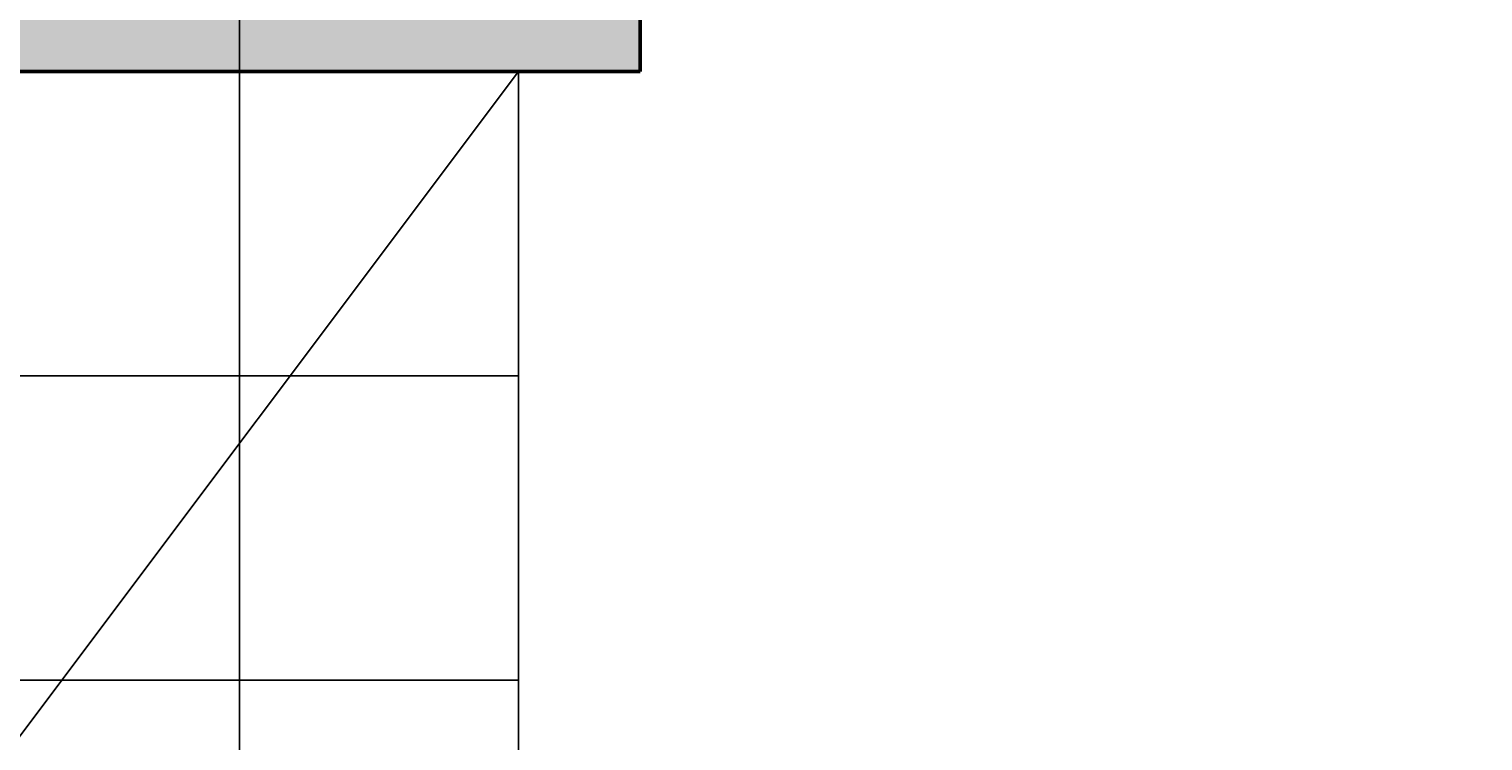
# Model space of a CAD drawing. Units: inches. Extents: x 2231 to 2461, y 2045 to 2455.
# Tile 7 of 95: x 2279 to 2326, y 2099 to 2122. Entities that reach past the tile are written whole.
import ezdxf

# ---------------------------------------------------------------- set-up
doc = ezdxf.new("R2010")
doc.units = ezdxf.units.IN
for name, color, linetype, lineweight in [('A-ANNO-DIMS', 2, 'Continuous', 18), ('A-FLOR-EVTR', 8, 'Continuous', 25), ('A-WALL', 7, 'Continuous', 50)]:
    doc.layers.add(name, color=color, linetype=linetype, lineweight=lineweight)
doc.layers.add('A-WALL-PATT', color=18, linetype='Continuous', lineweight=13, true_color=0x000000)
doc.styles.get("Standard").update_dxf_attribs({"font": 'arial.ttf'})
doc.dimstyles.get("Standard").update_dxf_attribs({"dimtxt": 0.18, "dimasz": 0.18, "dimexe": 0.18, "dimexo": 0.0625, "dimgap": 0.09, "dimtad": 0, "dimtih": 1, "dimtoh": 1, "dimdec": 4, "dimzin": 0, "dimdsep": 46, "dimtxsty": 'Standard', "dimcen": 0.09, "dimadec": 0, "dimazin": 0, "dimtfac": 1, "dimtdec": 4, "dimtofl": 0, "dimtmove": 0, "dimatfit": 3, "dimfxl": 1, "dimtolj": 1, "dimtzin": 0, "dimarcsym": 0})

# ---------------------------------------------------------------- blocks, each defined once
blk = doc.blocks.new('*D51')
at = {"layer": 'A-ANNO-DIMS', "color": 0, "lineweight": -2, "transparency": 16777216}
for p, q in [((2258.794, 2306.77), (2258.794, 2044.803)), ((2330.794, 2306.77), (2330.794, 2044.803)), ((2258.974, 2044.983), (2294.576, 2044.983)), ((2330.614, 2044.983), (2295.011, 2044.983))]:
    blk.add_line(p, q, dxfattribs=at)
at = {"layer": 'A-ANNO-DIMS', "color": 0, "transparency": 16777216}
for points in [[(2258.974, 2045.013), (2258.974, 2044.953), (2258.794, 2044.983)], [(2330.614, 2045.013), (2330.614, 2044.953), (2330.794, 2044.983)]]:
    blk.add_solid(points, dxfattribs=at)
at = {"layer": 'Defpoints', "color": 0, "transparency": 16777216}
for p in [(2258.794, 2306.833), (2330.794, 2306.833), (2330.794, 2044.983)]:
    blk.add_point(p, dxfattribs=at)
at = {"layer": 'A-ANNO-DIMS', "color": 0, "transparency": 16777216, "insert": (2294.794, 2044.983), "char_height": 0.18, "attachment_point": 5}
blk.add_mtext('\\A1;72', dxfattribs=at)
blk = doc.blocks.new('*D65')
at = {"layer": 'A-ANNO-DIMS', "color": 0, "lineweight": -2, "transparency": 16777216}
for p, q in [((2285.635, 2189.285), (2285.635, 2044.803)), ((2340.667, 2189.285), (2340.667, 2044.803)), ((2285.815, 2044.983), (2312.758, 2044.983)), ((2340.487, 2044.983), (2313.545, 2044.983))]:
    blk.add_line(p, q, dxfattribs=at)
at = {"layer": 'A-ANNO-DIMS', "color": 0, "transparency": 16777216}
for points in [[(2285.815, 2045.013), (2285.815, 2044.953), (2285.635, 2044.983)], [(2340.487, 2045.013), (2340.487, 2044.953), (2340.667, 2044.983)]]:
    blk.add_solid(points, dxfattribs=at)
at = {"layer": 'Defpoints', "color": 0, "transparency": 16777216}
for p in [(2285.635, 2189.348), (2340.667, 2189.348), (2340.667, 2044.983)]:
    blk.add_point(p, dxfattribs=at)
at = {"layer": 'A-ANNO-DIMS', "color": 0, "transparency": 16777216, "insert": (2313.151, 2044.983), "char_height": 0.18, "attachment_point": 5}
blk.add_mtext('\\A1;55.03', dxfattribs=at)

msp = doc.modelspace()

# ---------------------------------------------------------------- hatches: boundary and pattern name
at = {"layer": 'A-WALL-PATT'}
h = msp.add_hatch(color=256, dxfattribs=at)
h.dxf.hatch_style = 1
h.paths.add_polyline_path([(2441.7935, 2269.1535), (2432.7935, 2269.1535), (2432.7935, 2186.8328), (2396.7935, 2186.8328), (2396.7935, 2286.8328), (2394.7935, 2286.8328), (2394.7935, 2186.8328), (2334.7935, 2186.8328), (2334.7935, 2182.8328), (2432.7935, 2182.8328), (2432.7935, 2072.8328), (2416.6639, 2072.8328), (2416.6639, 2063.8328), (2441.7935, 2063.8328)])
h.paths.add_polyline_path([(2368.6639, 2072.8328), (2367.04, 2072.8328), (2330.7942, 2072.8328), (2330.7397, 2063.8328), (2368.6639, 2063.8328)])
h.paths.add_polyline_path([(2300.7392, 2068.3328), (2300.7392, 2072.8328), (2298.7935, 2072.8328), (2294.7935, 2072.8328), (2258.7935, 2072.8328), (2258.7935, 2120.8328), (2294.7935, 2120.8328), (2298.7935, 2120.8328), (2298.7935, 2128.8328), (2294.7935, 2128.8328), (2294.7935, 2124.8328), (2258.7935, 2124.8328), (2258.7935, 2182.8328), (2294.7935, 2182.8328), (2294.7935, 2174.8328), (2298.7935, 2174.8328), (2298.7935, 2182.8328), (2304.7935, 2182.8328), (2304.7935, 2186.8328), (2258.7935, 2186.8328), (2258.7935, 2221.999), (2249.7935, 2221.999), (2249.7935, 2063.8328), (2300.7392, 2063.8328)])
h.paths.add_polyline_path([(2391.9338, 2435.8328), (2333.82, 2435.8328), (2333.82, 2426.8328), (2368.7935, 2426.8328), (2368.7935, 2374.9508), (2368.7935, 2370.8328), (2372.3935, 2370.8328), (2372.7935, 2370.8328), (2372.7935, 2426.8328), (2391.9338, 2426.8328)])
h.paths.add_polyline_path([(2441.7935, 2435.8328), (2415.9338, 2435.8328), (2415.9338, 2426.8328), (2432.7935, 2426.8328), (2432.7935, 2334.8328), (2372.7935, 2334.8328), (2372.7935, 2346.8328), (2368.7935, 2346.8328), (2368.7935, 2306.8328), (2360.7935, 2306.8328), (2360.7935, 2302.8328), (2368.7935, 2302.8328), (2372.7935, 2302.8328), (2372.7935, 2330.8328), (2432.7935, 2330.8328), (2432.7935, 2317.1535), (2441.7935, 2317.1535)])
h.paths.add_polyline_path([(2285.82, 2435.8328), (2249.7935, 2435.8328), (2249.7935, 2269.999), (2258.7935, 2269.999), (2258.7935, 2302.8328), (2318.8168, 2302.8328), (2330.7935, 2302.8328), (2330.7935, 2306.8328), (2258.7935, 2306.8328), (2258.7935, 2426.8328), (2285.82, 2426.8328)])

# ---------------------------------------------------------------- linework, layer by layer
at = {"layer": 'A-FLOR-EVTR'}
for p, q in [((2258.7935, 2120.8328), (2294.7935, 2120.8328)), ((2294.7935, 2120.8328), (2258.7935, 2072.8328)), ((2294.7935, 2120.8328), (2294.7935, 2072.8328)), ((2258.7935, 2110.8328), (2294.7935, 2110.8328)), ((2258.7935, 2100.8328), (2294.7935, 2100.8328))]:
    msp.add_line(p, q, dxfattribs=at)
at = {"layer": 'A-WALL'}
for p, q in [((2298.7935, 2120.8328), (2298.7935, 2128.8328)), ((2258.7935, 2120.8328), (2294.7935, 2120.8328)), ((2294.7935, 2120.8328), (2298.7935, 2120.8328))]:
    msp.add_line(p, q, dxfattribs=at)

# ---------------------------------------------------------------- dimensions: what is measured, and where the dimension line sits
at = {"layer": 'A-ANNO-DIMS'}
for base, p1, p2, override, picture, middle in [((2330.7935, 2044.9825), (2258.7935, 2306.8328), (2330.7935, 2306.8328), {"dimdec": 0, "dimlfac": 1, "dimrnd": 0, "dimzin": 0, "dimdsep": 46, "dimlunit": 2}, '*D51', (2294.7935, 2044.9825)), ((2340.6673, 2044.9825), (2285.6353, 2189.3477), (2340.6673, 2189.3477), {"dimdec": 2, "dimlfac": 1, "dimrnd": 0, "dimzin": 0, "dimdsep": 46, "dimlunit": 2}, '*D65', (2313.1513, 2044.9825))]:
    dim = msp.add_linear_dim(base=base, p1=p1, p2=p2, dimstyle='Standard', override=override, dxfattribs=at)
    dim.commit()
    dim.dimension.update_dxf_attribs({"geometry": picture, "text_midpoint": middle})

doc.saveas('drawing.dxf')
